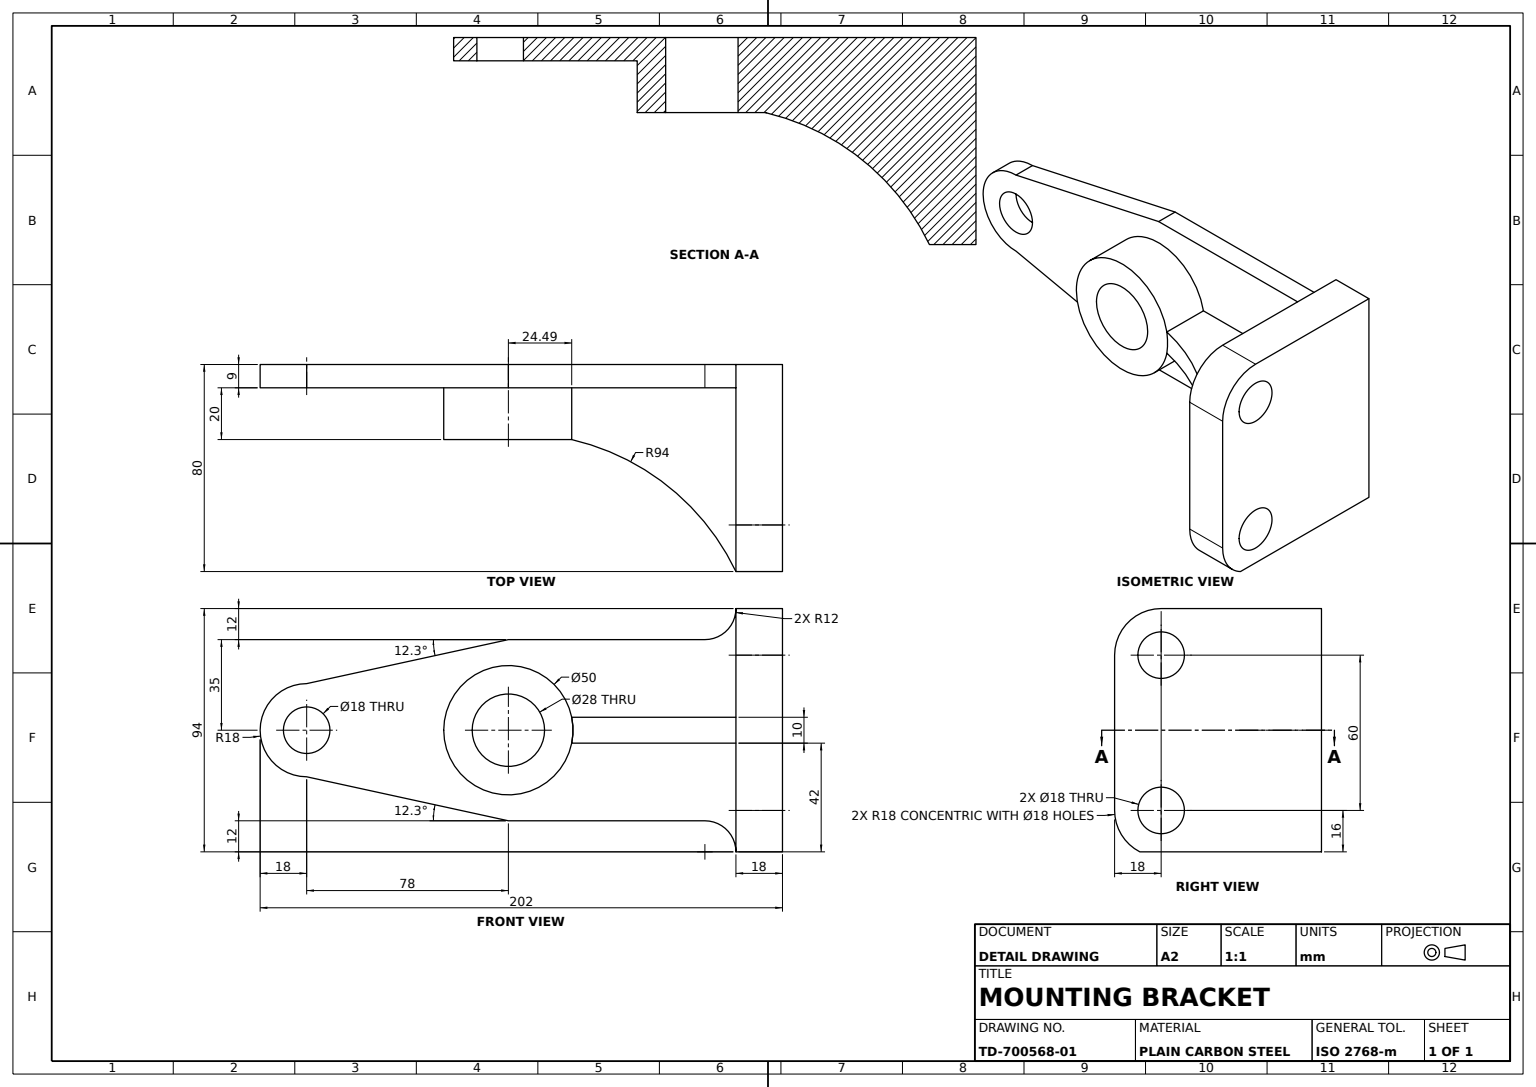
SolidWorks part; units mm, degrees
material "Plain Carbon Steel"
ref_plane "Front Plane" through (0, 0, 0) normal (0, 0, 1) x (1, 0, 0)
ref_plane "Top Plane" through (0, 0, 0) normal (0, 1, 0) x (1, 0, 0)
ref_plane "Right Plane" through (0, 0, 0) normal (1, 0, 0) x (0, 0, -1)
sketch "Arm Plate Sketch" plane through (0, 0, 0) normal (0, 0, 1) x (1, 0, 0)
  line L0 (0, 35) -> (-78, 18)
  line L4 (88, -47) -> (88, -48)
  line L5 (-88, 48) -> (88, -48) construction
  line L6 (-88, -48) -> (88, 48) construction
  line L7 (-78, -18) -> (0, -35)
  line L8 (88, 48) -> (88, -48)
  line L9 (0, 35) -> (76, 35)
  line L10 (0, -35) -> (76, -35)
  line L11 (25, 0) -> (62.8779, 0)
  line L12 (88, 47) -> (88, -47)
  circle A0 centre (-78, 0) radius 9
  circle A1 centre (-78, 0) radius 18
  circle A2 centre (0, 0) radius 25
  circle A3 centre (0, 0) radius 14
  arc A4 (76, -35) -> (88, -47) centre (76, -47) cw
  arc A5 (76, 35) -> (88, 47) centre (76, 47) ccw
  point P0 (0, 0)
  dimension "D2" = 36
  dimension "D3" = 18
  dimension "D4" = 50
  dimension "D5" = 28
  dimension "D9" = 12
  dimension "D1" = 176
  dimension "D6" = 78
  dimension "D7" = 35
  dimension "D8" = 35
  dimension "D10" = 96
  dimension "D11" = 37.8779
extrude "Arm Plate" add sketch "Arm Plate Sketch" along normal blind 9
sketch "Mounting Flange Sketch" plane through (88, 0, 0) normal (1, 0, 0) x (0, 0, -1)
  line L1 (-9, 47) -> (-62, 47)
  line L2 (-9, 47) -> (-9, -49)
  line L3 (-9, -49) -> (-62, -49)
  line L4 (-80, 29) -> (-80, -31)
  arc A0 (-62, -49) -> (-80, -31) centre (-62, -31) cw
  arc A1 (-62, 47) -> (-80, 29) centre (-62, 29) ccw
  circle A2 centre (-62, 29) radius 9
  circle A3 centre (-62, -31) radius 9
  point P7 (-80, -49)
  point P10 (-80, 47)
  dimension "D3" = 18
  dimension "D4" = 18
  dimension "D5" = 18
  dimension "D1" = 71
  dimension "D2" = 96
extrude "Mounting Flange" add sketch "Mounting Flange Sketch" along normal blind 18 separate body
sketch "Connecting Block Sketch" plane through (88, 0, 0) normal (1, 0, 0) x (0, 0, -1)
  line L1 (-9, 47) -> (0, 47)
  line L2 (-9, 47) -> (-9, -47)
  line L3 (-9, -47) -> (0, -47)
  line L4 (0, 47) -> (0, -47)
extrude "Connecting Block" add sketch "Connecting Block Sketch" along normal blind 18
sketch "Hub Boss Sketch" plane through (0, 0, 9) normal (0, 0, 1) x (1, 0, 0)
  circle A0 centre (0, 0) radius 25
  circle A1 centre (0, 0) radius 14
  dimension "D1" = 50
  dimension "D2" = 28
extrude "Hub Boss" add sketch "Hub Boss Sketch" along normal blind 20
sketch "Support Rib Sketch" plane through (0, 0, 9) normal (0, 0, 1) x (1, 0, 0)
  line L0 (88, 5) -> (88, -5)
  line L1 (88, -47) -> (88, 47) construction
  line L2 (88, 0) -> (88, 5)
  line L3 (88, 5) -> (24.4949, 5)
  line L4 (88, -5) -> (24.4949, -5)
  circle A0 centre (0, 0) radius 25 construction
  arc A1 (24.4949, 5) -> (24.4949, -5) centre (0, 0) cw
  line M4 (88, -47) -> (88, 47)
  circle M12 centre (0, 0) radius 25
  dimension "D1" = 10
extrude "Support Rib" add sketch "Support Rib Sketch" along normal blind 71 contours L4 L0 L3 M4 M12
sketch "Profile Trim Cut Sketch" plane through (0, -5, 0) normal (0, -1, 0) x (1, 0, 0)
  line L0 (88, 80) -> (24.4949, 80)
  line L1 (24.4949, 80) -> (24.4949, 29)
  arc A0 (24.4949, 29) -> (88, 80) centre (3.1989, 120.5559) ccw
  dimension "D1" = 94
extrude "Profile Trim Cut" cut sketch "Profile Trim Cut Sketch" against normal through all
sketch "Flange Cut Sketch" plane through (0, 0, 9) normal (0, 0, -1) x (-1, 0, 0)
  line L1 (-106, -47) -> (-88, -47)
  line L2 (-106, -47) -> (-106, -49)
  line L3 (-106, -49) -> (-88, -49)
  line L4 (-88, -47) -> (-88, -49)
extrude "Flange Cut" cut sketch "Flange Cut Sketch" against normal through all
